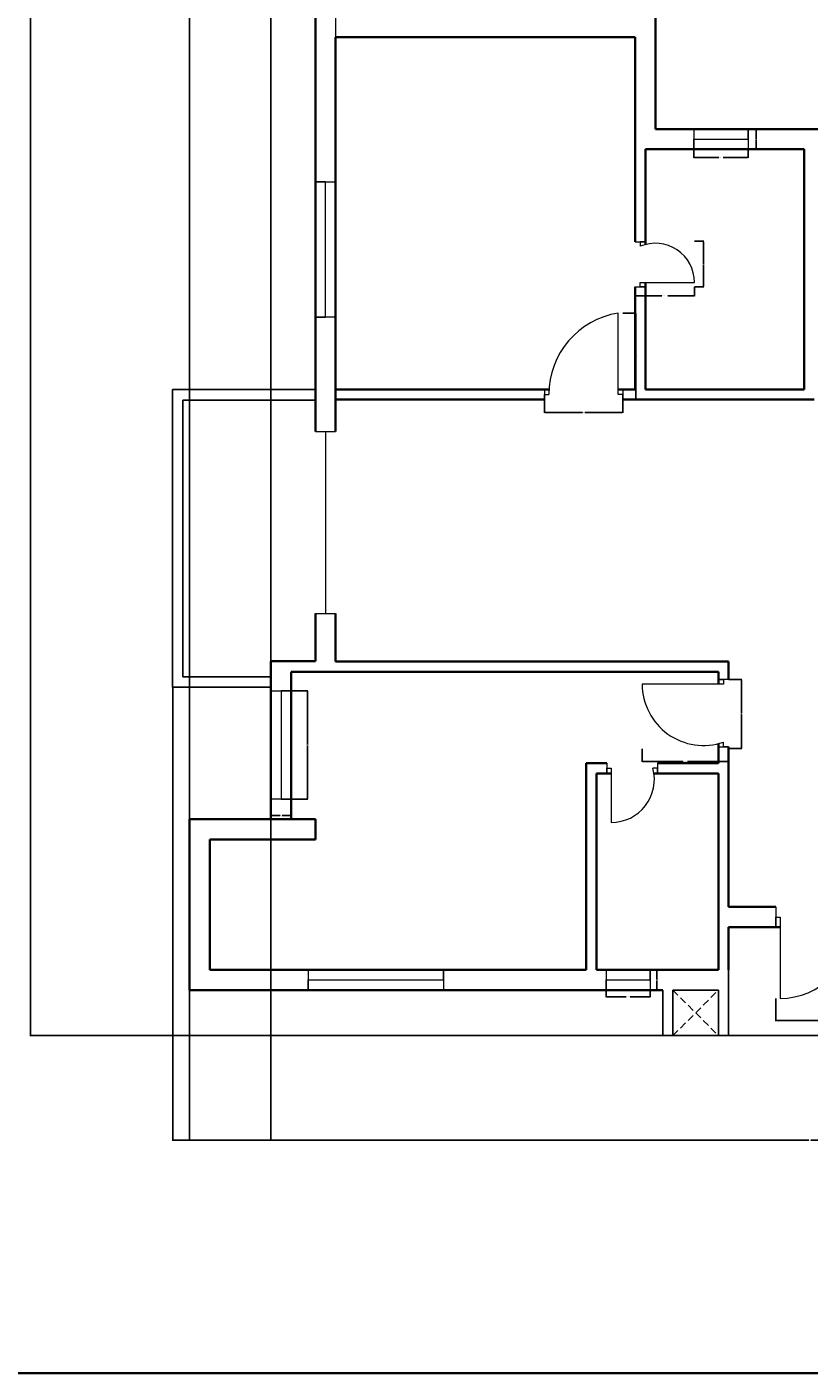
# Model space of a CAD drawing. Units: inches. Extents: x 2296 to 3812, y -1531 to 2564.
# Tile 6 of 10: x 3013 to 3359, y 1124 to 1720. Entities that reach past the tile are written whole.
import ezdxf

# ---------------------------------------------------------------- set-up
doc = ezdxf.new("R2010")
doc.units = ezdxf.units.IN
doc.linetypes.add('HIDDEN2', pattern=[4.7625, 3.175, -1.5875])
for name, color, linetype, lineweight in [('A-ANNO-DIMS', 2, 'Continuous', 18), ('A-ANNO-TTLB', 7, 'Continuous', 35), ('A-DOOR', 3, 'Continuous', 18), ('A-FLOR-HRAL', 7, 'Continuous', 25), ('A-GLAZ', 4, 'Continuous', 18), ('A-SECT-PROJ', 8, 'Continuous', 13), ('A-WALL', 7, 'Continuous', 35), ('A-WALL-HIDN', 8, 'HIDDEN2', 18)]:
    doc.layers.add(name, color=color, linetype=linetype, lineweight=lineweight)
doc.styles.get("Standard").update_dxf_attribs({"font": 'arial.ttf'})
doc.dimstyles.get("Standard").update_dxf_attribs({"dimtxt": 0.18, "dimasz": 0.18, "dimexe": 0.18, "dimexo": 0.0625, "dimgap": 0.09, "dimtad": 0, "dimtih": 1, "dimtoh": 1, "dimdec": 4, "dimzin": 0, "dimdsep": 46, "dimtxsty": 'Standard', "dimcen": 0.09, "dimadec": 0, "dimazin": 0, "dimtfac": 1, "dimtdec": 4, "dimtofl": 0, "dimtmove": 0, "dimatfit": 3, "dimfxl": 1, "dimtolj": 1, "dimtzin": 0, "dimarcsym": 0})

# ---------------------------------------------------------------- blocks, each defined once
blk = doc.blocks.new('DOOR-BEDROOM-36-WS')
for p, q in [((32.71, 2.25), (32.71, 38.25)), ((0, 4.5), (0, 0)), ((0, 0), (0, 2.25)), ((0, 2.25), (2, 2.25)), ((34.71, 2.25), (32.71, 2.25)), ((34.71, 4.5), (34.71, 0)), ((34.71, 0), (34.71, 2.25))]:
    blk.add_line(p, q)
blk.add_arc((38.45, 2.25), 36.46, 99.06194, 180)
blk = doc.blocks.new('DOOR-BATH-24-SW')
for p, q in [((0, 26.25), (0, 21.75)), ((0, 21.75), (0, 24)), ((0, 24), (2, 24)), ((2, 24), (2, 0)), ((22.44, 24), (20.44, 24)), ((22.44, 26.25), (22.44, 21.75)), ((22.44, 21.75), (22.44, 24))]:
    blk.add_line(p, q)
blk.add_arc((2, 19.08), 19.08, 270, 14.93359)
blk = doc.blocks.new('DOOR-BEDROOM-36-SW')
for p, q in [((36, 27.71), (0, 27.71)), ((38.25, 29.71), (33.75, 29.71)), ((33.75, 29.71), (36, 29.71)), ((36, 29.71), (36, 27.71)), ((36, 0), (36, 2)), ((33.75, 0), (38.25, 0)), ((38.25, 0), (36, 0))]:
    blk.add_line(p, q)
blk.add_arc((27.18, 27.71), 27.18, 180, 288.93127)
blk = doc.blocks.new('DOOR-BALCONY-PAIR-S')
for p, q in [((0, 40.5), (0, 31.5)), ((0, 31.5), (0, 36)), ((0, 36), (2, 36)), ((2, 36), (2, 0)), ((65.68, 36), (63.68, 36)), ((63.68, 36), (63.68, 0)), ((65.68, 40.5), (65.68, 31.5)), ((65.68, 31.5), (65.68, 36))]:
    blk.add_line(p, q)
for centre, radius, start, end in [((2, 31.87), 31.87, 270, 359.32793), ((65.8, 31.86), 31.93, 180.64039, 266.18908)]:
    blk.add_arc(centre, radius, start, end)
blk = doc.blocks.new('DOOR-BATH-24-WS')
for p, q in [((0, 20), (4.5, 20)), ((4.5, 20), (2.25, 20)), ((2.25, 20), (2.25, 18)), ((2.25, 0), (2.25, 2)), ((2.25, 2), (26.25, 2)), ((0, 0), (4.5, 0)), ((4.5, 0), (2.25, 0))]:
    blk.add_line(p, q)
blk.add_arc((8.92, 2), 17.33, 0, 112.62699)
blk = doc.blocks.new('WIN-60-JAMB-A')
for p, q in [((0, 60), (9, 60)), ((9, 60), (4.5, 60)), ((4.5, 60), (4.5, 0)), ((9, 0), (0, 0)), ((4.5, 0), (9, 0))]:
    blk.add_line(p, q)
blk = doc.blocks.new('WIN-48-BEDROOM-SW')
for p, q in [((0, 48), (9, 48)), ((9, 48), (4.5, 48)), ((4.5, 48), (4.5, 0)), ((9, 0), (0, 0)), ((4.5, 0), (9, 0))]:
    blk.add_line(p, q)
blk = doc.blocks.new('WIN-24-SHAFT-S')
for p, q in [((0, 9), (0, 0)), ((24, 4.5), (24, 9)), ((24, 9), (24, 0)), ((0, 0), (0, 4.5)), ((0, 4.5), (0, 4.5)), ((0, 4.5), (24, 4.5))]:
    blk.add_line(p, q)
blk = doc.blocks.new('WIN-60-SILL')
for p, q in [((0, 9), (0, 0)), ((60, 4.5), (60, 9)), ((60, 9), (60, 0)), ((0, 0), (0, 4.5)), ((0, 4.5), (60, 4.5))]:
    blk.add_line(p, q)
blk = doc.blocks.new('WIN-20-VENT')
for p, q in [((0, 9), (0, 0)), ((19.57, 4.5), (19.57, 9)), ((19.57, 9), (19.57, 0)), ((0, 0), (0, 4.5)), ((0, 4.5), (0, 4.5)), ((0, 4.5), (19.57, 4.5)), ((19.57, 0), (19.57, 0))]:
    blk.add_line(p, q)
blk = doc.blocks.new('GLAZ-BALCONY-S')
for p, q in [((0, 80.52), (9, 80.52)), ((4.5, 80.52), (4.5, 0)), ((0, 0), (9, 0))]:
    blk.add_line(p, q)
blk = doc.blocks.new('*D75')
at = {"layer": 'A-ANNO-DIMS', "color": 0, "lineweight": -2, "transparency": 16777216}
for p, q in [((3277.03, 1593.41), (3282.88, 1593.41)), ((3282.7, 1593.23), (3282.7, 1574.47)), ((3282.7, 1555.34), (3282.7, 1574.1)), ((3277.03, 1555.16), (3282.88, 1555.16))]:
    blk.add_line(p, q, dxfattribs=at)
at = {"layer": 'A-ANNO-DIMS', "color": 0, "transparency": 16777216}
for points in [[(3282.67, 1593.23), (3282.73, 1593.23), (3282.7, 1593.41)], [(3282.67, 1555.34), (3282.73, 1555.34), (3282.7, 1555.16)]]:
    blk.add_solid(points, dxfattribs=at)
at = {"layer": 'Defpoints', "color": 0, "transparency": 16777216}
for p in [(3276.97, 1593.41), (3282.7, 1593.41), (3276.97, 1555.16)]:
    blk.add_point(p, dxfattribs=at)
at = {"layer": 'A-ANNO-DIMS', "color": 0, "transparency": 16777216, "insert": (3282.7, 1574.28), "char_height": 0.18, "attachment_point": 5}
blk.add_mtext('\\A1;DOOR 38 TYP.', dxfattribs=at)
blk = doc.blocks.new('*D76')
at = {"layer": 'A-ANNO-DIMS', "color": 0, "lineweight": -2, "transparency": 16777216}
for p, q in [((3242.25, 1555.1), (3242.25, 1549.24)), ((3276.97, 1555.1), (3276.97, 1549.24)), ((3242.43, 1549.42), (3259.08, 1549.42)), ((3276.79, 1549.42), (3260.14, 1549.42))]:
    blk.add_line(p, q, dxfattribs=at)
at = {"layer": 'A-ANNO-DIMS', "color": 0, "transparency": 16777216}
for points in [[(3242.43, 1549.45), (3242.43, 1549.39), (3242.25, 1549.42)], [(3276.79, 1549.45), (3276.79, 1549.39), (3276.97, 1549.42)]]:
    blk.add_solid(points, dxfattribs=at)
at = {"layer": 'Defpoints', "color": 0, "transparency": 16777216}
for p in [(3242.25, 1555.16), (3276.97, 1555.16), (3276.97, 1549.42)]:
    blk.add_point(p, dxfattribs=at)
at = {"layer": 'A-ANNO-DIMS', "color": 0, "transparency": 16777216, "insert": (3259.61, 1549.42), "char_height": 0.18, "attachment_point": 5}
blk.add_mtext('\\A1;35 TYP.', dxfattribs=at)
blk = doc.blocks.new('*D85')
at = {"layer": 'A-ANNO-DIMS', "color": 0, "lineweight": -2, "transparency": 16777216}
for p, q in [((3285.59, 1400.5), (3285.59, 1394.65)), ((3323.84, 1400.5), (3323.84, 1394.65)), ((3285.77, 1394.83), (3303.78, 1394.83)), ((3323.66, 1394.83), (3305.65, 1394.83))]:
    blk.add_line(p, q, dxfattribs=at)
at = {"layer": 'A-ANNO-DIMS', "color": 0, "transparency": 16777216}
for points in [[(3285.77, 1394.86), (3285.77, 1394.8), (3285.59, 1394.83)], [(3323.66, 1394.86), (3323.66, 1394.8), (3323.84, 1394.83)]]:
    blk.add_solid(points, dxfattribs=at)
at = {"layer": 'Defpoints', "color": 0, "transparency": 16777216}
for p in [(3285.59, 1400.56), (3323.84, 1400.56), (3323.84, 1394.83)]:
    blk.add_point(p, dxfattribs=at)
at = {"layer": 'A-ANNO-DIMS', "color": 0, "transparency": 16777216, "insert": (3304.72, 1394.83), "char_height": 0.18, "attachment_point": 5}
blk.add_mtext('\\A1;DOOR 38 TYP.', dxfattribs=at)
blk = doc.blocks.new('*D86')
at = {"layer": 'A-ANNO-DIMS', "color": 0, "lineweight": -2, "transparency": 16777216}
for p, q in [((3323.9, 1431.12), (3329.76, 1431.12)), ((3329.58, 1430.94), (3329.58, 1416.03)), ((3329.58, 1400.74), (3329.58, 1415.66)), ((3323.9, 1400.56), (3329.76, 1400.56))]:
    blk.add_line(p, q, dxfattribs=at)
at = {"layer": 'A-ANNO-DIMS', "color": 0, "transparency": 16777216}
for points in [[(3329.55, 1430.94), (3329.61, 1430.94), (3329.58, 1431.12)], [(3329.55, 1400.74), (3329.61, 1400.74), (3329.58, 1400.56)]]:
    blk.add_solid(points, dxfattribs=at)
at = {"layer": 'Defpoints', "color": 0, "transparency": 16777216}
for p in [(3323.84, 1431.12), (3329.58, 1431.12), (3323.84, 1400.56)]:
    blk.add_point(p, dxfattribs=at)
at = {"layer": 'A-ANNO-DIMS', "color": 0, "transparency": 16777216, "insert": (3329.58, 1415.84), "char_height": 0.18, "attachment_point": 5}
blk.add_mtext('\\A1;31 TYP.', dxfattribs=at)
blk = doc.blocks.new('*D87')
at = {"layer": 'A-ANNO-DIMS', "color": 0, "lineweight": -2, "transparency": 16777216}
for p, q in [((3344.71, 1289.87), (3344.71, 1279.9)), ((3410.39, 1289.87), (3410.39, 1279.9)), ((3344.89, 1280.08), (3376.7, 1280.08)), ((3410.21, 1280.08), (3378.4, 1280.08))]:
    blk.add_line(p, q, dxfattribs=at)
at = {"layer": 'A-ANNO-DIMS', "color": 0, "transparency": 16777216}
for points in [[(3344.89, 1280.11), (3344.89, 1280.05), (3344.71, 1280.08)], [(3410.21, 1280.11), (3410.21, 1280.05), (3410.39, 1280.08)]]:
    blk.add_solid(points, dxfattribs=at)
at = {"layer": 'Defpoints', "color": 0, "transparency": 16777216}
for p in [(3344.71, 1289.93), (3410.39, 1289.93), (3410.39, 1280.08)]:
    blk.add_point(p, dxfattribs=at)
at = {"layer": 'A-ANNO-DIMS', "color": 0, "transparency": 16777216, "insert": (3377.55, 1280.08), "char_height": 0.18, "attachment_point": 5}
blk.add_mtext('\\A1;PAIR 66 TYP.', dxfattribs=at)
blk = doc.blocks.new('*D89')
at = {"layer": 'A-ANNO-DIMS', "color": 0, "lineweight": -2, "transparency": 16777216}
for p, q in [((3282.49, 1604.93), (3282.49, 1600.88)), ((3308.74, 1604.93), (3308.74, 1600.88)), ((3282.67, 1601.06), (3294.31, 1601.06)), ((3308.56, 1601.06), (3296.92, 1601.06))]:
    blk.add_line(p, q, dxfattribs=at)
at = {"layer": 'A-ANNO-DIMS', "color": 0, "transparency": 16777216}
for points in [[(3282.67, 1601.09), (3282.67, 1601.03), (3282.49, 1601.06)], [(3308.56, 1601.09), (3308.56, 1601.03), (3308.74, 1601.06)]]:
    blk.add_solid(points, dxfattribs=at)
at = {"layer": 'Defpoints', "color": 0, "transparency": 16777216}
for p in [(3282.49, 1604.99), (3308.74, 1604.99), (3308.74, 1601.06)]:
    blk.add_point(p, dxfattribs=at)
at = {"layer": 'A-ANNO-DIMS', "color": 0, "transparency": 16777216, "insert": (3295.61, 1601.06), "char_height": 0.18, "attachment_point": 5}
blk.add_mtext('\\A1;BATH DOOR 26 TYP.', dxfattribs=at)
blk = doc.blocks.new('*D90')
at = {"layer": 'A-ANNO-DIMS', "color": 0, "lineweight": -2, "transparency": 16777216}
for p, q in [((3308.8, 1625.22), (3312.86, 1625.22)), ((3312.68, 1625.04), (3312.68, 1615.29)), ((3312.68, 1605.17), (3312.68, 1614.93)), ((3308.8, 1604.99), (3312.86, 1604.99))]:
    blk.add_line(p, q, dxfattribs=at)
at = {"layer": 'A-ANNO-DIMS', "color": 0, "transparency": 16777216}
for points in [[(3312.65, 1625.04), (3312.71, 1625.04), (3312.68, 1625.22)], [(3312.65, 1605.17), (3312.71, 1605.17), (3312.68, 1604.99)]]:
    blk.add_solid(points, dxfattribs=at)
at = {"layer": 'Defpoints', "color": 0, "transparency": 16777216}
for p in [(3308.74, 1625.22), (3312.68, 1625.22), (3308.74, 1604.99)]:
    blk.add_point(p, dxfattribs=at)
at = {"layer": 'A-ANNO-DIMS', "color": 0, "transparency": 16777216, "insert": (3312.68, 1615.11), "char_height": 0.18, "attachment_point": 5}
blk.add_mtext('\\A1;20 TYP.', dxfattribs=at)
blk = doc.blocks.new('*D103')
at = {"layer": 'A-ANNO-DIMS', "color": 0, "lineweight": -2, "transparency": 16777216}
for p, q in [((3130.22, 1426.17), (3137.54, 1426.17)), ((3137.36, 1425.99), (3137.36, 1402.35)), ((3137.36, 1378.35), (3137.36, 1401.98)), ((3130.22, 1378.17), (3137.54, 1378.17))]:
    blk.add_line(p, q, dxfattribs=at)
at = {"layer": 'A-ANNO-DIMS', "color": 0, "transparency": 16777216}
for points in [[(3137.33, 1425.99), (3137.39, 1425.99), (3137.36, 1426.17)], [(3137.33, 1378.35), (3137.39, 1378.35), (3137.36, 1378.17)]]:
    blk.add_solid(points, dxfattribs=at)
at = {"layer": 'Defpoints', "color": 0, "transparency": 16777216}
for p in [(3130.16, 1426.17), (3137.36, 1426.17), (3130.16, 1378.17)]:
    blk.add_point(p, dxfattribs=at)
at = {"layer": 'A-ANNO-DIMS', "color": 0, "transparency": 16777216, "insert": (3137.36, 1402.17), "char_height": 0.18, "attachment_point": 5}
blk.add_mtext('\\A1;WINDOW 48 TYP.', dxfattribs=at)
blk = doc.blocks.new('*D104')
at = {"layer": 'A-ANNO-DIMS', "color": 0, "lineweight": -2, "transparency": 16777216}
for p, q in [((3121.16, 1378.1), (3121.16, 1370.79)), ((3130.16, 1378.1), (3130.16, 1370.79)), ((3121.34, 1370.97), (3125.2, 1370.97)), ((3129.98, 1370.97), (3126.12, 1370.97))]:
    blk.add_line(p, q, dxfattribs=at)
at = {"layer": 'A-ANNO-DIMS', "color": 0, "transparency": 16777216}
for points in [[(3121.34, 1371), (3121.34, 1370.94), (3121.16, 1370.97)], [(3129.98, 1371), (3129.98, 1370.94), (3130.16, 1370.97)]]:
    blk.add_solid(points, dxfattribs=at)
at = {"layer": 'Defpoints', "color": 0, "transparency": 16777216}
for p in [(3121.16, 1378.17), (3130.16, 1378.17), (3130.16, 1370.97)]:
    blk.add_point(p, dxfattribs=at)
at = {"layer": 'A-ANNO-DIMS', "color": 0, "transparency": 16777216, "insert": (3125.66, 1370.97), "char_height": 0.18, "attachment_point": 5}
blk.add_mtext('\\A1;9 TYP.', dxfattribs=at)
blk = doc.blocks.new('*D107')
at = {"layer": 'A-ANNO-DIMS', "color": 0, "lineweight": -2, "transparency": 16777216}
for p, q in [((3308.47, 1665.89), (3308.47, 1662.17)), ((3332.47, 1665.89), (3332.47, 1662.17)), ((3308.65, 1662.35), (3319.57, 1662.35)), ((3332.29, 1662.35), (3321.38, 1662.35))]:
    blk.add_line(p, q, dxfattribs=at)
at = {"layer": 'A-ANNO-DIMS', "color": 0, "transparency": 16777216}
for points in [[(3308.65, 1662.38), (3308.65, 1662.32), (3308.47, 1662.35)], [(3332.29, 1662.38), (3332.29, 1662.32), (3332.47, 1662.35)]]:
    blk.add_solid(points, dxfattribs=at)
at = {"layer": 'Defpoints', "color": 0, "transparency": 16777216}
for p in [(3308.47, 1665.95), (3332.47, 1665.95), (3332.47, 1662.35)]:
    blk.add_point(p, dxfattribs=at)
at = {"layer": 'A-ANNO-DIMS', "color": 0, "transparency": 16777216, "insert": (3320.47, 1662.35), "char_height": 0.18, "attachment_point": 5}
blk.add_mtext('\\A1;VENT 24 TYP.', dxfattribs=at)
blk = doc.blocks.new('*D108')
at = {"layer": 'A-ANNO-DIMS', "color": 0, "lineweight": -2, "transparency": 16777216}
for p, q in [((3332.54, 1674.95), (3336.25, 1674.95)), ((3336.07, 1674.77), (3336.07, 1670.63)), ((3336.07, 1666.13), (3336.07, 1670.27)), ((3332.54, 1665.95), (3336.25, 1665.95))]:
    blk.add_line(p, q, dxfattribs=at)
at = {"layer": 'A-ANNO-DIMS', "color": 0, "transparency": 16777216}
for points in [[(3336.04, 1674.77), (3336.1, 1674.77), (3336.07, 1674.95)], [(3336.04, 1666.13), (3336.1, 1666.13), (3336.07, 1665.95)]]:
    blk.add_solid(points, dxfattribs=at)
at = {"layer": 'Defpoints', "color": 0, "transparency": 16777216}
for p in [(3332.47, 1674.95), (3336.07, 1674.95), (3332.47, 1665.95)]:
    blk.add_point(p, dxfattribs=at)
at = {"layer": 'A-ANNO-DIMS', "color": 0, "transparency": 16777216, "insert": (3336.07, 1670.45), "char_height": 0.18, "attachment_point": 5}
blk.add_mtext('\\A1;9 TYP.', dxfattribs=at)
blk = doc.blocks.new('*D117')
at = {"layer": 'A-ANNO-DIMS', "color": 0, "lineweight": -2, "transparency": 16777216}
for p, q in [((3269.62, 1293.54), (3269.62, 1290.49)), ((3269.8, 1290.67), (3278.5, 1290.67)), ((3289, 1290.67), (3280.31, 1290.67)), ((3289.18, 1293.54), (3289.18, 1290.49))]:
    blk.add_line(p, q, dxfattribs=at)
at = {"layer": 'A-ANNO-DIMS', "color": 0, "transparency": 16777216}
for points in [[(3269.8, 1290.7), (3269.8, 1290.64), (3269.62, 1290.67)], [(3289, 1290.7), (3289, 1290.64), (3289.18, 1290.67)]]:
    blk.add_solid(points, dxfattribs=at)
at = {"layer": 'Defpoints', "color": 0, "transparency": 16777216}
for p in [(3269.62, 1293.6), (3289.18, 1293.6), (3289.18, 1290.67)]:
    blk.add_point(p, dxfattribs=at)
at = {"layer": 'A-ANNO-DIMS', "color": 0, "transparency": 16777216, "insert": (3279.4, 1290.67), "char_height": 0.18, "attachment_point": 5}
blk.add_mtext('\\A1;VENT 20 TYP.', dxfattribs=at)
blk = doc.blocks.new('*D118')
at = {"layer": 'A-ANNO-DIMS', "color": 0, "lineweight": -2, "transparency": 16777216}
for p, q in [((3289.25, 1302.6), (3292.3, 1302.6)), ((3292.12, 1302.42), (3292.12, 1298.28)), ((3292.12, 1293.78), (3292.12, 1297.92)), ((3289.25, 1293.6), (3292.3, 1293.6))]:
    blk.add_line(p, q, dxfattribs=at)
at = {"layer": 'A-ANNO-DIMS', "color": 0, "transparency": 16777216}
for points in [[(3292.09, 1302.42), (3292.15, 1302.42), (3292.12, 1302.6)], [(3292.09, 1293.78), (3292.15, 1293.78), (3292.12, 1293.6)]]:
    blk.add_solid(points, dxfattribs=at)
at = {"layer": 'Defpoints', "color": 0, "transparency": 16777216}
for p in [(3289.18, 1302.6), (3292.12, 1302.6), (3289.18, 1293.6)]:
    blk.add_point(p, dxfattribs=at)
at = {"layer": 'A-ANNO-DIMS', "color": 0, "transparency": 16777216, "insert": (3292.12, 1298.1), "char_height": 0.18, "attachment_point": 5}
blk.add_mtext('\\A1;9 TYP.', dxfattribs=at)
blk = doc.blocks.new('*D129')
at = {"layer": 'A-ANNO-DIMS', "color": 0, "lineweight": -2, "transparency": 16777216}
for p, q in [((3641.99, 1498.34), (3641.99, 1226.9)), ((3077.66, 1427.77), (3077.66, 1226.9)), ((3077.84, 1227.08), (3359.43, 1227.08)), ((3641.81, 1227.08), (3360.22, 1227.08))]:
    blk.add_line(p, q, dxfattribs=at)
at = {"layer": 'A-ANNO-DIMS', "color": 0, "transparency": 16777216}
for points in [[(3077.84, 1227.11), (3077.84, 1227.05), (3077.66, 1227.08)], [(3641.81, 1227.11), (3641.81, 1227.05), (3641.99, 1227.08)]]:
    blk.add_solid(points, dxfattribs=at)
at = {"layer": 'Defpoints', "color": 0, "transparency": 16777216}
for p in [(3641.99, 1498.4), (3077.66, 1427.84), (3641.99, 1227.08)]:
    blk.add_point(p, dxfattribs=at)
at = {"layer": 'A-ANNO-DIMS', "color": 0, "transparency": 16777216, "insert": (3359.83, 1227.08), "char_height": 0.18, "attachment_point": 5}
blk.add_mtext('\\A1;564.3', dxfattribs=at)
blk = doc.blocks.new('*D130')
at = {"layer": 'A-ANNO-DIMS', "color": 0, "lineweight": -2, "transparency": 16777216}
for p, q in [((3313.1, 2175.03), (3014.48, 2175.03)), ((3014.66, 2174.85), (3014.66, 1724.41)), ((3014.66, 1273.61), (3014.66, 1724.05)), ((3319.28, 1273.43), (3014.48, 1273.43))]:
    blk.add_line(p, q, dxfattribs=at)
at = {"layer": 'A-ANNO-DIMS', "color": 0, "transparency": 16777216}
for points in [[(3014.63, 2174.85), (3014.69, 2174.85), (3014.66, 2175.03)], [(3014.63, 1273.61), (3014.69, 1273.61), (3014.66, 1273.43)]]:
    blk.add_solid(points, dxfattribs=at)
at = {"layer": 'Defpoints', "color": 0, "transparency": 16777216}
for p in [(3014.66, 2175.03), (3313.16, 2175.03), (3319.34, 1273.43)]:
    blk.add_point(p, dxfattribs=at)
at = {"layer": 'A-ANNO-DIMS', "color": 0, "transparency": 16777216, "insert": (3014.66, 1724.23), "char_height": 0.18, "attachment_point": 5}
blk.add_mtext('\\A1;901.6', dxfattribs=at)
blk = doc.blocks.new('*D143')
at = {"layer": 'A-ANNO-DIMS', "color": 0, "lineweight": -2, "transparency": 16777216}
for p, q in [((3085.16, 2086.2), (3085.16, 1226.9)), ((3121.16, 2086.2), (3121.16, 1226.9)), ((3085.34, 1227.08), (3102.94, 1227.08)), ((3120.98, 1227.08), (3103.38, 1227.08))]:
    blk.add_line(p, q, dxfattribs=at)
at = {"layer": 'A-ANNO-DIMS', "color": 0, "transparency": 16777216}
for points in [[(3085.34, 1227.11), (3085.34, 1227.05), (3085.16, 1227.08)], [(3120.98, 1227.11), (3120.98, 1227.05), (3121.16, 1227.08)]]:
    blk.add_solid(points, dxfattribs=at)
at = {"layer": 'Defpoints', "color": 0, "transparency": 16777216}
for p in [(3085.16, 2086.26), (3121.16, 2086.26), (3121.16, 1227.08)]:
    blk.add_point(p, dxfattribs=at)
at = {"layer": 'A-ANNO-DIMS', "color": 0, "transparency": 16777216, "insert": (3103.16, 1227.08), "char_height": 0.18, "attachment_point": 5}
blk.add_mtext('\\A1;36', dxfattribs=at)

msp = doc.modelspace()

# ---------------------------------------------------------------- linework, layer by layer
at = {"layer": 'A-ANNO-TTLB'}
msp.add_lwpolyline([(2296.1257, 2564.2989), (3812.4193, 2564.2989), (3812.4193, 1124.0028), (2296.1257, 1124.0028)], close=True, dxfattribs=at)
at = {"layer": 'A-FLOR-HRAL'}
for p, q in [((3077.6588, 1559.6578), (3077.6588, 1427.8367)), ((3082.1588, 1559.6578), (3077.6588, 1559.6578)), ((3082.1588, 1559.6578), (3140.8418, 1559.6578)), ((3082.1588, 1432.3367), (3082.1588, 1554.9294)), ((3140.8418, 1554.9294), (3082.1588, 1554.9294)), ((3121.1588, 1432.3367), (3082.1588, 1432.3367)), ((3121.1588, 1431.0117), (3121.1588, 1435.5117)), ((3121.1588, 1427.8367), (3121.1588, 1432.3367)), ((3077.6588, 1427.8367), (3121.1588, 1427.8367)), ((3323.8418, 1302.6012), (3323.8418, 1273.434)), ((3294.6651, 1293.6012), (3294.6651, 1273.434)), ((3299.1651, 1293.6012), (3319.3418, 1293.6012)), ((3299.1651, 1273.434), (3299.1651, 1293.6012)), ((3319.3418, 1293.6012), (3319.3418, 1273.434)), ((3294.6651, 1273.434), (3299.1651, 1273.434)), ((3319.3418, 1273.434), (3323.8418, 1273.434)), ((3437.6588, 1273.434), (3323.8418, 1273.434))]:
    msp.add_line(p, q, dxfattribs=at)
at = {"layer": 'A-SECT-PROJ'}
for p, q in [((3140.8418, 1901.6355), (3140.8418, 1540.9318)), ((3149.8418, 1901.6355), (3149.8418, 1540.9318))]:
    msp.add_line(p, q, dxfattribs=at)
at = {"layer": 'A-WALL'}
for p, q in [((3140.8418, 1901.6355), (3140.8418, 1540.9318)), ((3291.4894, 1780.1578), (3291.4894, 1715.6578)), ((3149.8418, 1715.6578), (3267.3064, 1715.6578)), ((3149.8418, 1715.6578), (3149.8418, 1555.1578)), ((3267.3064, 1715.6578), (3282.4894, 1715.6578)), ((3282.4894, 1715.6578), (3282.4894, 1624.9927)), ((3291.4894, 1715.6578), (3291.4894, 1674.9485)), ((3291.4894, 1674.9485), (3366.2648, 1674.9485)), ((3286.9894, 1623.7542), (3286.9894, 1665.9485)), ((3357.2648, 1665.9485), (3286.9894, 1665.9485)), ((3357.2648, 1665.9485), (3357.2648, 1599.9948)), ((3282.4894, 1604.9949), (3282.4894, 1559.6578)), ((3286.9894, 1559.6578), (3286.9894, 1606.9949)), ((3357.2648, 1599.9948), (3357.2648, 1559.6578)), ((3149.8418, 1559.6578), (3244.3228, 1559.6578)), ((3282.4894, 1559.6578), (3274.9666, 1559.6578)), ((3357.2648, 1559.6578), (3286.9894, 1559.6578)), ((3149.8418, 1555.1578), (3242.2533, 1555.1578)), ((3149.8418, 1555.1578), (3149.8418, 1540.9318)), ((3276.9666, 1555.1578), (3282.4894, 1555.1578)), ((3282.4894, 1555.1578), (3286.9894, 1555.1578)), ((3361.7116, 1555.1578), (3286.9894, 1555.1578)), ((3140.8418, 1460.4105), (3140.8418, 1439.3482)), ((3149.8418, 1460.4105), (3149.8418, 1439.1012)), ((3121.1588, 1439.3482), (3121.1588, 1434.6012)), ((3140.8418, 1439.3482), (3121.1588, 1439.3482)), ((3265.3418, 1439.1012), (3149.8418, 1439.1012)), ((3265.3418, 1439.1012), (3323.8418, 1439.1012)), ((3323.8418, 1439.1012), (3323.8418, 1434.6012)), ((3121.1588, 1434.6012), (3121.1588, 1369.3709)), ((3130.1588, 1434.6012), (3140.8418, 1434.6012)), ((3140.8418, 1434.6012), (3130.1588, 1434.6012)), ((3130.1588, 1434.6012), (3130.1588, 1369.3709)), ((3140.8418, 1434.6012), (3260.8418, 1434.6012)), ((3265.3418, 1434.6012), (3260.8418, 1434.6012)), ((3319.3418, 1434.6012), (3265.3418, 1434.6012)), ((3319.3418, 1429.1229), (3319.3418, 1434.6012)), ((3323.8418, 1434.6012), (3323.8418, 1431.1229)), ((3319.3418, 1394.1012), (3319.3418, 1402.747)), ((3323.8418, 1401.4117), (3323.8418, 1394.1012)), ((3260.8418, 1394.1012), (3260.8418, 1302.6012)), ((3269.9038, 1394.1012), (3260.8418, 1394.1012)), ((3265.3418, 1302.6012), (3265.3418, 1389.6012)), ((3271.9038, 1389.6012), (3265.3418, 1389.6012)), ((3319.3418, 1389.6012), (3290.7989, 1389.6012)), ((3319.3418, 1394.1012), (3292.3418, 1394.1012)), ((3319.3418, 1302.6012), (3319.3418, 1389.6012)), ((3323.8418, 1330.434), (3323.8418, 1394.1012)), ((3323.8418, 1389.6012), (3323.8418, 1394.1012)), ((3323.8418, 1330.434), (3323.8418, 1389.6012)), ((3085.1588, 1369.3709), (3085.1588, 1293.6012)), ((3140.8418, 1369.3709), (3085.1588, 1369.3709)), ((3140.8418, 1360.3709), (3140.8418, 1369.3709)), ((3094.1588, 1302.6012), (3094.1588, 1360.3709)), ((3094.1588, 1360.3709), (3140.8418, 1360.3709)), ((3344.7145, 1330.434), (3323.8418, 1330.434)), ((3323.8418, 1302.6012), (3323.8418, 1321.434)), ((3323.8418, 1302.6012), (3323.8418, 1321.434)), ((3323.8418, 1321.434), (3346.7145, 1321.434)), ((3094.1588, 1302.6012), (3260.8418, 1302.6012)), ((3094.1588, 1302.6012), (3260.8418, 1302.6012)), ((3265.3418, 1302.6012), (3319.3418, 1302.6012)), ((3265.3418, 1302.6012), (3319.3418, 1302.6012)), ((3085.1588, 1293.6012), (3294.6651, 1293.6012))]:
    msp.add_line(p, q, dxfattribs=at)
at = {"layer": 'A-WALL-HIDN'}
for p, q in [((3299.1651, 1273.434), (3319.3418, 1293.6012)), ((3299.1651, 1293.6012), (3319.3418, 1273.434))]:
    msp.add_line(p, q, dxfattribs=at)

# ---------------------------------------------------------------- block references
at = {"layer": 'A-DOOR'}
for name, p in [('DOOR-BATH-24-WS', (3282.4894, 1604.995)), ('DOOR-BEDROOM-36-WS', (3242.2534, 1555.158)), ('DOOR-BEDROOM-36-SW', (3285.5914, 1401.412)), ('DOOR-BATH-24-SW', (3269.9034, 1367.851)), ('DOOR-BALCONY-PAIR-S', (3344.7144, 1289.934))]:
    msp.add_blockref(name, p, dxfattribs=at)
at = {"layer": 'A-GLAZ'}
for name, p in [('WIN-24-SHAFT-S', (3308.4734, 1665.948)), ('GLAZ-BALCONY-S', (3140.8414, 1460.411)), ('WIN-48-BEDROOM-SW', (3121.1584, 1378.167)), ('WIN-60-SILL', (3137.623, 1293.601)), ('WIN-20-VENT', (3269.6194, 1293.601))]:
    msp.add_blockref(name, p, dxfattribs=at)
at = {"layer": 'A-GLAZ', "rotation": 180}
msp.add_blockref('WIN-60-JAMB-A', (3149.842, 1651.6229), dxfattribs=at)

# ---------------------------------------------------------------- dimensions: what is measured, and where the dimension line sits
at = {"layer": 'A-ANNO-DIMS'}
dim = msp.add_linear_dim(base=(3014.6644, 2175.0276), p1=(3319.3418, 1273.434), p2=(3313.1588, 2175.0276), angle=90, dimstyle='Standard', override={"dimdec": 1, "dimlfac": 1, "dimrnd": 0, "dimzin": 0, "dimdsep": 46, "dimlunit": 2}, dxfattribs=at)
dim.commit()
dim.dimension.update_dxf_attribs({"geometry": '*D130', "text_midpoint": (3014.6644, 1724.2308)})
for base, p1, p2, override, picture, middle in [((3121.1588, 1227.084), (3085.1588, 2086.2649), (3121.1588, 2086.2649), {"dimdec": 0, "dimlfac": 1, "dimrnd": 0, "dimzin": 0, "dimdsep": 46, "dimlunit": 2}, '*D143', (3103.1588, 1227.084)), ((3641.9944, 1227.084), (3077.6588, 1427.8367), (3641.9944, 1498.4048), {"dimdec": 1, "dimlfac": 1, "dimrnd": 0, "dimzin": 0, "dimdsep": 46, "dimlunit": 2}, '*D129', (3359.8266, 1227.084))]:
    dim = msp.add_linear_dim(base=base, p1=p1, p2=p2, dimstyle='Standard', override=override, dxfattribs=at)
    dim.commit()
    dim.dimension.update_dxf_attribs({"geometry": picture, "text_midpoint": middle})
for base, p1, p2, text, picture, middle in [((3336.0735, 1674.9485), (3332.4735, 1665.9485), (3332.4735, 1674.9485), '<> TYP.', '*D108', (3336.0735, 1670.4485)), ((3312.6769, 1625.2224), (3308.7394, 1604.9949), (3308.7394, 1625.2224), '<> TYP.', '*D90', (3312.6769, 1615.1086)), ((3282.7041, 1593.4078), (3276.9666, 1555.1578), (3276.9666, 1593.4078), 'DOOR <> TYP.', '*D75', (3282.7041, 1574.2828)), ((3329.5793, 1431.1229), (3323.8418, 1400.5636), (3323.8418, 1431.1229), '<> TYP.', '*D86', (3329.5793, 1415.8432)), ((3137.3588, 1426.167), (3130.1588, 1378.167), (3130.1588, 1426.167), 'WINDOW <> TYP.', '*D103', (3137.3588, 1402.167)), ((3292.1194, 1302.6012), (3289.1846, 1293.6012), (3289.1846, 1302.6012), '<> TYP.', '*D118', (3292.1194, 1298.1012))]:
    dim = msp.add_linear_dim(base=base, p1=p1, p2=p2, angle=90, text=text, dimstyle='Standard', override={"dimdec": 0, "dimlfac": 1, "dimrnd": 0, "dimzin": 0, "dimdsep": 46, "dimlunit": 2}, dxfattribs=at)
    dim.commit()
    dim.dimension.update_dxf_attribs({"geometry": picture, "text_midpoint": middle})
for base, p1, p2, text, picture, middle in [((3332.4735, 1662.3485), (3308.4735, 1665.9485), (3332.4735, 1665.9485), 'VENT <> TYP.', '*D107', (3320.4735, 1662.3485)), ((3308.7394, 1601.0574), (3282.4894, 1604.9949), (3308.7394, 1604.9949), 'BATH DOOR <> TYP.', '*D89', (3295.6144, 1601.0574)), ((3276.9666, 1549.4203), (3242.2533, 1555.1578), (3276.9666, 1555.1578), '<> TYP.', '*D76', (3259.61, 1549.4203)), ((3323.8418, 1394.8261), (3285.5918, 1400.5636), (3323.8418, 1400.5636), 'DOOR <> TYP.', '*D85', (3304.7168, 1394.8261)), ((3130.1588, 1370.967), (3121.1588, 1378.167), (3130.1588, 1378.167), '<> TYP.', '*D104', (3125.6588, 1370.967)), ((3289.1846, 1290.6665), (3269.6198, 1293.6012), (3289.1846, 1293.6012), 'VENT <> TYP.', '*D117', (3279.4022, 1290.6665)), ((3410.3896, 1280.0827), (3344.7145, 1289.934), (3410.3896, 1289.934), 'PAIR <> TYP.', '*D87', (3377.5521, 1280.0827))]:
    dim = msp.add_linear_dim(base=base, p1=p1, p2=p2, text=text, dimstyle='Standard', override={"dimdec": 0, "dimlfac": 1, "dimrnd": 0, "dimzin": 0, "dimdsep": 46, "dimlunit": 2}, dxfattribs=at)
    dim.commit()
    dim.dimension.update_dxf_attribs({"geometry": picture, "text_midpoint": middle})

doc.saveas('drawing.dxf')
